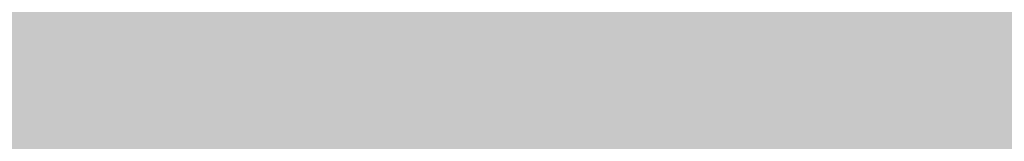
# Model space of a CAD drawing. Units: inches. Extents: x 2083 to 3317, y 1141 to 2115.
# Tile 154 of 256: x 3126.946713 to 3126.955939, y 1263.262504 to 1263.263648. Entities that reach past the tile are written whole.
import ezdxf

# ---------------------------------------------------------------- set-up
doc = ezdxf.new("R2010")
doc.units = ezdxf.units.IN
doc.layers.add('A-ANNO-DIMS', color=2, linetype='Continuous', lineweight=18)
doc.layers.add('A-WALL-PATT', color=251, linetype='Continuous', lineweight=13, true_color=0x636466)
doc.styles.get("Standard").update_dxf_attribs({"font": 'arial.ttf'})
doc.dimstyles.new('ISO-25', dxfattribs={"dimtxt": 12, "dimasz": 12, "dimexe": 1.25, "dimexo": 0.625, "dimtad": 1, "dimlunit": 3, "dimtxsty": 'Standard', "dimcen": 2.5, "dimadec": 0, "dimazin": 0, "dimtfac": 1, "dimtmove": 0, "dimatfit": 3, "dimfxl": 1, "dimarcsym": 0})

# ---------------------------------------------------------------- blocks, each defined once
blk = doc.blocks.new('*D26')
at = {"layer": 'A-ANNO-DIMS', "color": 0, "lineweight": -2, "transparency": 16777216}
for p, q in [((3088.985844, 1274.915092), (3088.985844, 1270.9519631)), ((3111.2400366, 1274.915092), (3111.2400366, 1270.9519631)), ((3076.985844, 1272.2019631), (2840.262447, 1272.2019631)), ((3111.2400366, 1272.2019631), (3088.985844, 1272.2019631)), ((3123.2400366, 1272.2019631), (3135.2400366, 1272.2019631))]:
    blk.add_line(p, q, dxfattribs=at)
at = {"layer": 'A-ANNO-DIMS', "color": 0, "transparency": 16777216}
for points in [[(3076.985844, 1274.2019631), (3076.985844, 1270.2019631), (3088.985844, 1272.2019631)], [(3123.2400366, 1274.2019631), (3123.2400366, 1270.2019631), (3111.2400366, 1272.2019631)]]:
    blk.add_solid(points, dxfattribs=at)
at = {"layer": 'Defpoints', "color": 0, "transparency": 16777216}
for p in [(3088.985844, 1275.540092), (3111.2400366, 1275.540092), (3088.985844, 1272.2019631)]:
    blk.add_point(p, dxfattribs=at)
at = {"layer": 'A-ANNO-DIMS', "color": 0, "transparency": 16777216, "insert": (2952.6241455, 1279.0316016), "char_height": 12, "attachment_point": 5}
blk.add_mtext('NIGHTSTAND 1\'-10 1/2" TYP.', dxfattribs=at)

msp = doc.modelspace()

# ---------------------------------------------------------------- hatches: boundary and pattern name
at = {"layer": 'A-WALL-PATT'}
h = msp.add_hatch(color=256, dxfattribs=at)
h.dxf.hatch_style = 1
h.paths.add_polyline_path([(3126.9597832, 2020.7613601), (2748.9597832, 2020.7613601), (2604.9597832, 2020.7613601), (2226.9597832, 2020.7613601), (2226.9597832, 1702.7613601), (2466.9597832, 1702.7613601), (2466.9597832, 1582.7613601), (2418.9597832, 1582.7613601), (2418.9597832, 1477.7613601), (2226.9597832, 1477.7613601), (2226.9597832, 1263.2613601), (2544.9597832, 1263.2613601), (2544.9597832, 1411.7613601), (2604.9597832, 1411.7613601), (2685.9597832, 1411.7613601), (2685.9597832, 1420.7613601), (2604.9597832, 1420.7613601), (2604.9597832, 1573.7613601), (2604.9597832, 1702.7613601), (2604.9597832, 2011.7613601), (2748.9597832, 2011.7613601), (2748.9597832, 1702.7613601), (2862.9597832, 1702.7613601), (2862.9597832, 1621.7613601), (2871.9597832, 1621.7613601), (2871.9597832, 1702.7613601), (2883.9597832, 1702.7613601), (2883.9597832, 1706.9394595, -0.026459), (2883.9597832, 1711.7613601), (2757.9597832, 1711.7613601), (2757.9597832, 1807.7613601), (2787.9597832, 1807.7613601), (2787.9597832, 1812.2613601), (2757.9597832, 1812.2613601), (2757.9597832, 2011.7613601), (2877.9597832, 2011.7613601), (2877.9597832, 1812.2613601), (2847.9597832, 1812.2613601), (2847.9597832, 1807.7613601), (2889.8357425, 1807.7613601), (2889.8357425, 1812.2613601), (2882.4597832, 1812.2613601), (2882.4597832, 2011.7613601), (3117.9597832, 2011.7613601), (3117.9597832, 1812.2613601), (2937.8357425, 1812.2613601), (2937.8357425, 1807.7613601), (2995.7097832, 1807.7613601), (2995.7097832, 1796.1176655), (3000.2097832, 1796.1176655), (3000.2097832, 1807.7613601), (3117.9597832, 1807.7613601), (3117.9597832, 1711.7613601), (3000.2097832, 1711.7613601), (3000.2097832, 1760.1176655), (2998.5727047, 1760.1176655, -0.020711), (2995.7097832, 1760.1176655), (2995.7097832, 1711.7613601), (2931.9597832, 1711.7613601), (2931.9597832, 1702.7613601), (3126.9597832, 1702.7613601)])
h.paths.add_polyline_path([(2471.4597832, 2011.7613601), (2471.4597832, 1810.0113601), (2462.7169357, 1810.0113601), (2462.7169357, 1805.5113601), (2505.9597832, 1805.5113601), (2505.9597832, 1810.0113601), (2475.9597832, 1810.0113601), (2475.9597832, 2011.7613601), (2595.9597832, 2011.7613601), (2595.9597832, 1810.0113601), (2565.9597832, 1810.0113601), (2565.9597832, 1805.5113601), (2595.9597832, 1805.5113601), (2595.9597832, 1711.7613601), (2235.9597832, 1711.7613601), (2235.9597832, 1805.5113601), (2353.7097832, 1805.5113601), (2353.7097832, 1796.0541624), (2358.2097832, 1796.0541624), (2358.2097832, 1805.5113601), (2414.7169357, 1805.5113601), (2414.7169357, 1810.0113601), (2235.9597832, 1810.0113601), (2235.9597832, 2011.7613601)], flags=16)
h.paths.add_polyline_path([(2270.2047343, 1994.6100082), (2270.2047343, 1970.6100082), (2246.2047343, 1970.6100082), (2246.2047343, 1994.6100082)], flags=0)
edge = h.paths.add_edge_path(flags=0)
edge.add_ellipse((2332.027391, 1899.7981761), major_axis=(-3.0429938, 3.0429938), ratio=0.16825245, start_angle=-161.3321656, end_angle=-156.3071136, ccw=False)
edge.add_ellipse((2333.0820373, 1898.7435297), major_axis=(-1.0546463, 1.0546463), ratio=0.453532097, start_angle=-123.371019, end_angle=-94.1591066)
edge = h.paths.add_edge_path(flags=0)
edge.add_ellipse((2332.027391, 1968.8762897), major_axis=(3.0429938, 3.0429938), ratio=0.16825245, start_angle=18.6678344, end_angle=23.6928864)
edge.add_spline(control_points=[(2332.9255964, 1970.6911045), (2332.2267681, 1970.3360997), (2330.8937087, 1969.6589054), (2328.4130803, 1970.9321376), (2327.2039345, 1967.7487119), (2324.7095965, 1969.9555886), (2322.5328223, 1967.012354), (2320.0128462, 1971.2958124), (2317.6803077, 1968.1578449), (2316.0405263, 1967.1020468), (2315.4269045, 1966.8096022)], knot_values=[0, 0, 0, 0, 2.267059, 4.324559, 6.685584, 8.878641, 11.121502, 14.300359, 17.755284, 19.732645, 19.732645, 19.732645, 19.732645], degree=3, periodic=0)
edge.add_ellipse((2332.027391, 1968.8762897), major_axis=(3.0429938, 3.0429938), ratio=0.16825245, start_angle=18.6678344, end_angle=23.6928864, ccw=False)
edge.add_ellipse((2333.0820373, 1969.930936), major_axis=(1.0546463, 1.0546463), ratio=0.453532097, start_angle=56.628981, end_angle=85.8408934, ccw=False)
edge = h.paths.add_edge_path(flags=0)
edge.add_spline(control_points=[(2296.4282874, 1967.9879081), (2293.6278045, 1965.3363137), (2287.7036238, 1959.727094), (2299.7438601, 1949.9956993), (2294.5325909, 1935.6685275), (2290.5732281, 1920.6035119), (2293.3941244, 1909.9736911), (2296.1854073, 1904.9665431)], knot_values=[0.099185, 0.099185, 0.099185, 0.099185, 0.345301, 0.619822, 0.982653, 1.386093, 1.810555, 1.810555, 1.810555, 1.810555], degree=3, periodic=0)
edge.add_spline(control_points=[(2296.1854073, 1904.9665431), (2297.3835817, 1902.6193002), (2298.0009694, 1901.9493116), (2298.5529698, 1901.4681549)], knot_values=[0.006246, 0.006246, 0.006246, 0.006246, 0.055476, 0.055476, 0.055476, 0.055476], degree=3, periodic=0)
edge.add_spline(control_points=[(2298.5529698, 1901.4681549), (2297.2586121, 1900.9232238), (2295.2252939, 1900.2321257), (2293.0602287, 1900.6142053), (2292.1014227, 1900.788415), (2292.0895776, 1900.790568)], knot_values=[0.312835, 0.312835, 0.312835, 0.312835, 0.40178, 0.474987, 0.475903, 0.475903, 0.475903, 0.475903], degree=3, periodic=0)
edge.add_arc((2292.7936464, 1904.6641088), 3.9370079, 215.4208969, 259.6981795, ccw=False)
edge.add_spline(control_points=[(2289.5853139, 1902.3823039), (2289.4766524, 1902.5350874), (2289.3684805, 1902.6880353), (2289.2608648, 1902.8411699)], knot_values=[0.102872, 0.102872, 0.102872, 0.102872, 0.116896, 0.116896, 0.116896, 0.116896], degree=3, periodic=0)
edge.add_spline(control_points=[(2289.2608648, 1902.8411699), (2288.6866042, 1902.5501922), (2287.6400477, 1902.0199025), (2285.8813368, 1901.8739536), (2283.8529717, 1901.5043521), (2281.7199871, 1899.7105375), (2278.4669913, 1899.492942), (2276.1571361, 1901.8832022), (2272.2589526, 1899.8040711), (2267.7776054, 1901.8431828), (2262.2438819, 1900.1840326), (2257.414927, 1901.7820606), (2254.318374, 1900.7261196), (2253.1782849, 1900.3373431)], knot_values=[0, 0, 0, 0, 1.907977, 3.477176, 5.261074, 7.972851, 11.680248, 13.717921, 16.939592, 22.789562, 27.502503, 33.595215, 37.145618, 37.145618, 37.145618, 37.145618], degree=3, periodic=0)
edge.add_line((2253.1782849, 1900.3373431), (2250.2442397, 1902.8411699))
edge.add_line((2250.2442397, 1902.8411699), (2250.2442397, 1965.8332959))
edge.add_line((2250.2442397, 1965.8332959), (2253.1782849, 1968.3371226))
edge.add_spline(control_points=[(2253.1782849, 1968.3371226), (2254.318374, 1967.9483462), (2257.414927, 1966.8924051), (2262.2438819, 1968.4904332), (2267.7776054, 1966.8312829), (2271.5267301, 1968.5372172), (2273.8759143, 1967.8282895), (2274.2067012, 1967.7276424)], knot_values=[0, 0, 0, 0, 0.09018, 0.244935, 0.364644, 0.513233, 0.537855, 0.537855, 0.537855, 0.537855], degree=3, periodic=0)
edge.add_arc((2274.3528869, 1963.7933495), 3.9370079, 72.0511336, 92.1279492, ccw=False)
edge.add_arc((2281.2969331, 1985.2300027), 18.5962982, 252.05113361, 288.56572166)
edge.add_arc((2292.3167172, 1956.0288805), 12.6460805, 71.02678788, 113.77821843, ccw=False)
edge = h.paths.add_edge_path(flags=0)
edge.add_spline(control_points=[(2274.8994147, 1951.8561946), (2275.066156, 1951.6165924), (2275.2326866, 1951.3765878), (2275.3979871, 1951.1358545)], knot_values=[1.409916, 1.409916, 1.409916, 1.409916, 1.43159, 1.43159, 1.43159, 1.43159], degree=3, periodic=0)
edge.add_spline(control_points=[(2275.3979871, 1951.1358545), (2275.7921055, 1950.5618854), (2276.1792311, 1949.9837745), (2276.5455462, 1949.3971029)], knot_values=[1.358238, 1.358238, 1.358238, 1.358238, 1.409916, 1.409916, 1.409916, 1.409916], degree=3, periodic=0)
edge.add_line((2276.5455462, 1949.3971029), (2277.437289, 1947.8621847))
edge.add_spline(control_points=[(2277.437289, 1947.8621847), (2276.3038341, 1945.6731147), (2274.6396979, 1942.4268817), (2274.631615, 1938.0938998), (2272.7991237, 1930.8515498), (2274.3564261, 1943.8970461), (2275.9476814, 1947.9233558), (2276.5455462, 1949.3971029)], knot_values=[0.005632, 0.005632, 0.005632, 0.005632, 0.186014, 0.266002, 0.357087, 0.59639, 0.739732, 0.739732, 0.739732, 0.739732], degree=3, periodic=0)
edge.add_spline(control_points=[(2276.5455462, 1949.3971029), (2276.1792311, 1949.9837745), (2275.7921055, 1950.5618854), (2275.3979871, 1951.1358545)], knot_values=[1.358238, 1.358238, 1.358238, 1.358238, 1.409916, 1.409916, 1.409916, 1.409916], degree=3, periodic=0)
edge.add_spline(control_points=[(2275.3979871, 1951.1358545), (2274.9425002, 1950.0804523), (2274.2077604, 1948.0252718), (2273.9346018, 1944.8514774), (2272.4685341, 1937.6274891), (2273.4662155, 1945.6964663), (2274.7006154, 1951.0594725), (2274.8994147, 1951.8561946)], knot_values=[0.104364, 0.104364, 0.104364, 0.104364, 0.189636, 0.269624, 0.36071, 0.600013, 0.644622, 0.644622, 0.644622, 0.644622], degree=3, periodic=0)
h.paths.add_polyline_path([(2269.1675139, 1963.1275729, -0.357527), (2268.170633, 1960.9763695, -0.092561), (2268.170633, 1939.4363249, -0.357527), (2269.1675139, 1937.2851215, -0.357527), (2267.0163105, 1938.2820024, -0.164785), (2254.6855813, 1938.2820024, -0.357527), (2252.5343779, 1937.2851215, -0.357527), (2253.5312587, 1939.4363249, -0.092561), (2253.5312587, 1960.9763695, -0.357527), (2252.5343779, 1963.1275729, -0.357527), (2254.6855813, 1962.130692, -0.164785), (2267.0163105, 1962.130692, -0.357527)], flags=0)
h.paths.add_polyline_path([(2248.8740679, 1967.8017998), (2248.8740679, 1957.0277095), (2249.4577833, 1957.0277095), (2249.4577833, 1911.6467562), (2248.8740679, 1911.6467562), (2248.8740679, 1900.8726659), (2246.5118632, 1900.8726659, 0.197327), (2244.1496584, 1902.4568734), (2244.1496584, 1966.2175923, 0.197327), (2246.5118632, 1967.8017998)], flags=0)
h.paths.add_polyline_path([(2269.1675139, 1931.3893442, -0.357527), (2268.170633, 1929.2381408, -0.092561), (2268.170633, 1907.6980962, -0.357527), (2269.1675139, 1905.5468928, -0.357527), (2267.0163105, 1906.5437737, -0.164785), (2254.6855813, 1906.5437737, -0.357527), (2252.5343779, 1905.5468928, -0.357527), (2253.5312587, 1907.6980962, -0.092561), (2253.5312587, 1929.2381408, -0.357527), (2252.5343779, 1931.3893442, -0.357527), (2254.6855813, 1930.3924634, -0.164785), (2267.0163105, 1930.3924634, -0.357527)], flags=0)
edge = h.paths.add_edge_path(flags=0)
edge.add_spline(control_points=[(2276.1968578, 1906.7237016), (2276.1681442, 1909.0289278), (2276.1140492, 1913.371852), (2270.5984171, 1924.9249783), (2273.9051746, 1919.0127787), (2275.9217115, 1916.2620626), (2275.4745699, 1912.4021495), (2277.2578735, 1910.3806206), (2276.6960436, 1908.2250358), (2276.6462176, 1906.8130226), (2276.6178249, 1906.0084068)], knot_values=[0, 0, 0, 0, 8.61026, 16.221274, 18.843057, 23.804898, 27.440828, 29.356102, 31.203478, 33.650687, 33.650687, 33.650687, 33.650687], degree=3, periodic=0)
edge.add_spline(control_points=[(2276.6178249, 1906.0084068), (2276.6233131, 1905.6241436), (2276.4977381, 1904.6286608), (2275.4417789, 1903.8547251), (2274.9373144, 1903.0804497), (2274.8590804, 1902.8411699)], knot_values=[0.156488, 0.156488, 0.156488, 0.156488, 0.184398, 0.231376, 0.250598, 0.250598, 0.250598, 0.250598], degree=3, periodic=0)
edge.add_line((2274.8590804, 1902.8411699), (2276.50598, 1902.8411699))
edge.add_spline(control_points=[(2276.50598, 1902.8411699), (2276.7883084, 1903.0849395), (2277.6650711, 1904.1251958), (2278.2495378, 1904.340738), (2277.6538719, 1908.5273866), (2278.15567, 1906.2278078), (2278.100464, 1905.2859484), (2278.8466748, 1904.0690054), (2277.8567853, 1903.4149482), (2277.8741909, 1902.9910497), (2277.9035616, 1902.8411699)], knot_values=[0.059574, 0.059574, 0.059574, 0.059574, 0.080753, 0.103741, 0.16972, 0.176036, 0.207137, 0.240474, 0.262341, 0.27366, 0.27366, 0.27366, 0.27366], degree=3, periodic=0)
edge.add_line((2277.9035616, 1902.8411699), (2280.0298255, 1902.8411699))
edge.add_spline(control_points=[(2280.0298255, 1902.8411699), (2279.8882214, 1903.088398), (2279.4992571, 1903.9815512), (2280.1522839, 1905.9393491), (2278.103615, 1909.6577572), (2279.7623946, 1907.185285), (2280.3279002, 1904.8748608), (2280.4851086, 1903.4895904), (2281.4632687, 1903.2494323), (2281.7583431, 1902.9364967), (2281.8340361, 1902.8411699)], knot_values=[0.013856, 0.013856, 0.013856, 0.013856, 0.034874, 0.088867, 0.107879, 0.126738, 0.158714, 0.193757, 0.217487, 0.226722, 0.226722, 0.226722, 0.226722], degree=3, periodic=0)
edge.add_spline(control_points=[(2281.8340361, 1902.8411699), (2281.7875348, 1902.8267029), (2281.6470224, 1902.7829881), (2281.3955272, 1902.85949), (2281.088077, 1902.9852418), (2280.7206826, 1903.060902), (2280.3334513, 1903.0257257), (2280.1247668, 1902.898879), (2280.0298255, 1902.8411699)], knot_values=[0, 0, 0, 0, 0.14413, 0.435517, 0.749276, 1.153046, 1.548371, 1.878348, 1.878348, 1.878348, 1.878348], degree=3, periodic=0)
edge.add_line((2280.0298255, 1902.8411699), (2277.9035616, 1902.8411699))
edge.add_spline(control_points=[(2277.9035616, 1902.8411699), (2277.892855, 1902.7958553), (2277.865396, 1902.6796374), (2277.6074793, 1902.6874828), (2277.2740503, 1902.8006999), (2276.8379209, 1902.6197745), (2276.5838074, 1902.7892611), (2276.50598, 1902.8411699)], knot_values=[0, 0, 0, 0, 0.127189, 0.326199, 0.628009, 1.24357, 1.515331, 1.515331, 1.515331, 1.515331], degree=3, periodic=0)
edge.add_line((2276.50598, 1902.8411699), (2274.8590804, 1902.8411699))
edge.add_spline(control_points=[(2274.8590804, 1902.8411699), (2274.8144367, 1902.8985868), (2274.7251297, 1903.013446), (2274.4934765, 1903.1189684), (2274.2442854, 1902.9605386), (2273.9371207, 1903.1849416), (2273.6140395, 1902.9831428), (2273.4083164, 1902.8830449), (2273.322254, 1902.8411699)], knot_values=[0, 0, 0, 0, 0.21843, 0.436957, 0.687977, 0.990379, 1.398396, 1.69185, 1.69185, 1.69185, 1.69185], degree=3, periodic=0)
edge.add_spline(control_points=[(2273.322254, 1902.8411699), (2273.6167403, 1903.445692), (2274.2739977, 1904.5382529), (2276.0272387, 1904.5737017), (2276.2069634, 1906.5836372), (2276.1968578, 1906.7237016)], knot_values=[0.012227, 0.012227, 0.012227, 0.012227, 0.059472, 0.106218, 0.134458, 0.134458, 0.134458, 0.134458], degree=3, periodic=0)
h.paths.add_polyline_path([(2270.7760538, 1897.7898284), (2270.7760538, 1873.7898284), (2246.7760538, 1873.7898284), (2246.7760538, 1897.7898284)], flags=0)
h.paths.add_polyline_path([(2353.7097832, 1760.0050593), (2353.7097832, 1760.0541624), (2358.2097832, 1760.0541624, -0.033729)], flags=0)
h.paths.add_polyline_path([(2321.8191188, 1737.5291862), (2341.9953271, 1737.5291862, -0.414214), (2343.2032727, 1736.3212406), (2343.2032727, 1721.0205964, -0.414214), (2341.9953271, 1719.8126508), (2321.8191188, 1719.8126508, -0.414214), (2320.6111732, 1721.0205964), (2320.6111732, 1736.3212406, -0.414214)], flags=0)
h.paths.add_polyline_path([(2324.2350099, 1736.3212406), (2339.5794359, 1736.3212406, -0.414214), (2341.9953271, 1733.9053494), (2341.9953271, 1725.4497302, -0.414214), (2339.5794359, 1723.033839), (2333.6805885, 1723.033839), (2333.8453172, 1722.0454666, -0.870646), (2335.4253988, 1721.8258934, -0.767327), (2333.922694, 1721.4232449), (2331.2910241, 1721.4232449, -0.767327), (2329.7883193, 1721.8258934, -0.870646), (2331.3684009, 1722.0454666), (2331.5331296, 1723.033839), (2324.2350099, 1723.033839, -0.414214), (2321.8191188, 1725.4497302), (2321.8191188, 1733.9053494, -0.414214)], flags=0)
h.paths.add_polyline_path([(2570.4837892, 1928.6154443), (2589.6837892, 1928.6154443), (2590.1688286, 1928.6154443), (2590.1688286, 1904.9933971), (2570.4837892, 1904.9933971)], flags=0)
h.paths.add_polyline_path([(2574.4473242, 1927.2638215, -1), (2572.8288357, 1927.2638215, -1)], flags=0)
h.paths.add_polyline_path([(2573.0898665, 1926.9408768), (2573.925032, 1927.7760423), (2574.1477428, 1927.5533315), (2573.3125773, 1926.718166)], flags=0)
h.paths.add_polyline_path([(2578.7790648, 1919.7296175, -1), (2571.5916632, 1919.7296175, -1)], flags=0)
h.paths.add_polyline_path([(2578.385364, 1919.7296175, -1), (2571.985364, 1919.7296175, -1)], flags=0)
h.paths.add_polyline_path([(2331.5957638, 1729.4762156, -1), (2333.6179542, 1729.4762156, -1)], flags=0)
h.paths.add_polyline_path([(2578.0342282, 1927.2638215, -1), (2576.4157396, 1927.2638215, -1)], flags=0)
h.paths.add_polyline_path([(2576.6888513, 1927.5310886), (2576.9115621, 1927.7537993), (2577.7467276, 1926.9186339), (2577.5240168, 1926.6959231)], flags=0)
h.paths.add_polyline_path([(2578.1390648, 1909.8595388, -1), (2572.2316632, 1909.8595388, -1)], flags=0)
h.paths.add_polyline_path([(2577.745364, 1909.8595388, -1), (2572.625364, 1909.8595388, -1)], flags=0)
h.paths.add_polyline_path([(2583.7977179, 1927.2638215, -1), (2582.1792294, 1927.2638215, -1)], flags=0)
h.paths.add_polyline_path([(2582.7186487, 1927.7537993), (2583.5538142, 1926.9186339), (2583.3311034, 1926.6959231), (2582.4959379, 1927.5310886)], flags=0)
h.paths.add_polyline_path([(2582.4959379, 1927.5310886), (2582.7186487, 1927.7537993), (2583.5538142, 1926.9186339), (2583.3311034, 1926.6959231)], flags=0)
h.paths.add_polyline_path([(2587.7390648, 1920.5296175, -1), (2581.8316632, 1920.5296175, -1)], flags=0)
h.paths.add_polyline_path([(2587.345364, 1920.5296175, -1), (2582.225364, 1920.5296175, -1)], flags=0)
h.paths.add_polyline_path([(2587.3846219, 1927.2638215, -1), (2585.7661333, 1927.2638215, -1)], flags=0)
h.paths.add_polyline_path([(2586.0819925, 1926.9802469), (2586.917158, 1927.8154124), (2587.1398688, 1927.5927016), (2586.3047033, 1926.7575361)], flags=0)
h.paths.add_polyline_path([(2588.3790648, 1910.6595388, -1), (2581.1916632, 1910.6595388, -1)], flags=0)
h.paths.add_polyline_path([(2587.985364, 1910.6595388, -1), (2581.585364, 1910.6595388, -1)], flags=0)
h.paths.add_polyline_path([(2417.1677288, 1729.4778955), (2437.3439372, 1729.4778955, -0.414214), (2438.5518828, 1728.2699499), (2438.5518828, 1712.9693057, -0.414214), (2437.3439372, 1711.7613601), (2417.1677288, 1711.7613601, -0.414214), (2415.9597832, 1712.9693057), (2415.9597832, 1728.2699499, -0.414214)], flags=0)
h.paths.add_polyline_path([(2419.58362, 1728.2699499), (2434.928046, 1728.2699499, -0.414214), (2437.3439372, 1725.8540587), (2437.3439372, 1717.3984395, -0.414214), (2434.928046, 1714.9825483), (2429.0291985, 1714.9825483), (2429.1939273, 1713.9941758, -0.870646), (2430.7740089, 1713.7746027, -0.767327), (2429.2713041, 1713.3719542), (2426.6396342, 1713.3719542, -0.767327), (2425.1369294, 1713.7746027, -0.870646), (2426.717011, 1713.9941758), (2426.8817397, 1714.9825483), (2419.58362, 1714.9825483, -0.414214), (2417.1677288, 1717.3984395), (2417.1677288, 1725.8540587, -0.414214)], flags=0)
h.paths.add_polyline_path([(2419.58362, 1728.2699499), (2434.928046, 1728.2699499, -0.414214), (2437.3439372, 1725.8540587), (2437.3439372, 1717.3984395, -0.414214), (2434.928046, 1714.9825483), (2429.0291985, 1714.9825483), (2428.3581177, 1719.0090337), (2427.5528206, 1719.0090337), (2426.8817397, 1714.9825483), (2419.58362, 1714.9825483, -0.414214), (2417.1677288, 1717.3984395), (2417.1677288, 1725.8540587, -0.414214)], flags=0)
h.paths.add_polyline_path([(2426.9443739, 1721.4249248, -1), (2428.9665643, 1721.4249248, -1)], flags=0)
h.paths.add_polyline_path([(2475.9597832, 1702.7613601), (2595.9597832, 1702.7613601), (2595.9597832, 1582.7613601), (2475.9597832, 1582.7613601)], flags=16)
h.paths.add_polyline_path([(2427.9597832, 1573.7613601), (2595.9597832, 1573.7613601), (2595.9597832, 1468.7613601), (2595.9597832, 1420.7613601), (2384.4597832, 1420.7613601), (2384.4597832, 1468.7613601), (2427.9597832, 1468.7613601)], flags=16)
h.paths.add_polyline_path([(2379.9597832, 1468.7613601), (2379.9597832, 1420.7613601), (2235.9597832, 1420.7613601), (2235.9597832, 1468.7613601)], flags=16)
h.paths.add_polyline_path([(2317.8159962, 1466.695767), (2337.9922045, 1466.695767, -0.414214), (2339.2001501, 1465.4878214), (2339.2001501, 1450.1871771, -0.414214), (2337.9922045, 1448.9792315), (2317.8159962, 1448.9792315, -0.414214), (2316.6080506, 1450.1871771), (2316.6080506, 1465.4878214, -0.414214)], flags=0)
h.paths.add_polyline_path([(2320.2318874, 1465.4878214), (2335.5763133, 1465.4878214, -0.414214), (2337.9922045, 1463.0719302), (2337.9922045, 1454.616311, -0.414214), (2335.5763133, 1452.2004198), (2329.6774659, 1452.2004198), (2329.8421946, 1451.2120473, -0.870646), (2331.4222762, 1450.9924742, -0.767327), (2329.9195714, 1450.5898257), (2327.2879015, 1450.5898257, -0.767327), (2325.7851967, 1450.9924742, -0.870646), (2327.3652783, 1451.2120473), (2327.530007, 1452.2004198), (2320.2318874, 1452.2004198, -0.414214), (2317.8159962, 1454.616311), (2317.8159962, 1463.0719302, -0.414214)], flags=0)
h.paths.add_polyline_path([(2320.2318874, 1465.4878214), (2335.5763133, 1465.4878214, -0.414214), (2337.9922045, 1463.0719302), (2337.9922045, 1454.616311, -0.414214), (2335.5763133, 1452.2004198), (2329.6774659, 1452.2004198), (2329.006385, 1456.2269051), (2328.2010879, 1456.2269051), (2327.530007, 1452.2004198), (2320.2318874, 1452.2004198, -0.414214), (2317.8159962, 1454.616311), (2317.8159962, 1463.0719302, -0.414214)], flags=0)
h.paths.add_polyline_path([(2327.5926413, 1458.6427963, -1), (2329.6148317, 1458.6427963, -1)], flags=0)
h.paths.add_polyline_path([(2244.4117436, 1433.3404531), (2241.9209449, 1433.3404531, -0.414214), (2240.0178562, 1435.2435418), (2240.0178562, 1440.9528078, -0.414211), (2241.920925, 1442.8558965), (2244.4117436, 1442.8558965, -1.976472)], flags=0)
h.paths.add_polyline_path([(2245.3568884, 1434.3975358, -0.414214), (2245.3568884, 1441.7988138, -2.144098)], flags=0)
h.paths.add_polyline_path([(2535.9597832, 1416.2613601), (2535.9597832, 1272.2613601), (2235.9597832, 1272.2613601), (2235.9597832, 1416.2613601)], flags=16)
h.paths.add_polyline_path([(2260.1195614, 1384.2928413), (2260.1195614, 1362.0386487), (2237.8653688, 1362.0386487), (2237.8653688, 1384.2928413)], flags=0)
edge = h.paths.add_edge_path(flags=0)
edge.add_line((2318.2518466, 1362.0932983), (2318.1457968, 1362.0009726))
edge.add_ellipse((2317.4451158, 1360.4310442), major_axis=(2.8216404, 2.8216404), ratio=0.16825245, start_angle=18.6678344, end_angle=20.9481273, ccw=False)
edge.add_ellipse((2318.4230451, 1361.4089735), major_axis=(0.9779293, 0.9779293), ratio=0.453532097, start_angle=56.628981, end_angle=70.2262012, ccw=False)
edge = h.paths.add_edge_path(flags=0)
edge.add_line((2319.1073699, 1295.5710784), (2319.0150442, 1295.6771282))
edge.add_ellipse((2317.4451158, 1296.3778091), major_axis=(-2.8216404, 2.8216404), ratio=0.16825245, start_angle=-161.3321656, end_angle=-159.0518727, ccw=False)
edge.add_ellipse((2318.4230451, 1295.3998798), major_axis=(-0.9779293, 0.9779293), ratio=0.453532097, start_angle=-123.371019, end_angle=-109.7737988)
edge = h.paths.add_edge_path(flags=0)
edge.add_spline(control_points=[(2284.2103489, 1301.1702189), (2284.5806878, 1300.444719), (2284.8911891, 1299.8920243), (2285.159553, 1299.4610182)], knot_values=[0.039066, 0.039066, 0.039066, 0.039066, 0.055476, 0.055476, 0.055476, 0.055476], degree=3, periodic=0)
edge.add_line((2285.159553, 1299.4610182), (2284.2103489, 1301.1702189))
edge = h.paths.add_edge_path(flags=0)
edge.add_line((2280.4124579, 1297.2980125), (2283.3699905, 1297.0361216))
edge.add_line((2283.3699905, 1297.0361216), (2286.4056902, 1297.9263104))
edge.add_spline(control_points=[(2286.4056902, 1297.9263104), (2285.305487, 1297.4631193), (2284.3447774, 1297.1291508), (2283.3699905, 1297.0361216)], knot_values=[0.394369, 0.394369, 0.394369, 0.394369, 0.475903, 0.475903, 0.475903, 0.475903], degree=3, periodic=0)
edge.add_spline(control_points=[(2283.3699905, 1297.0361216), (2283.2813895, 1297.027666), (2282.316289, 1296.9573356), (2281.3125019, 1297.1344787), (2280.4234414, 1297.2960161), (2280.4124579, 1297.2980125)], knot_values=[0.312835, 0.312835, 0.312835, 0.312835, 0.320246, 0.393453, 0.394369, 0.394369, 0.394369, 0.394369], degree=3, periodic=0)
edge = h.paths.add_edge_path(flags=0)
edge.add_line((2284.4355615, 1359.6072854), (2280.4462909, 1355.328047))
edge.add_line((2280.4462909, 1355.328047), (2279.5799868, 1351.0177544))
edge.add_line((2279.5799868, 1351.0177544), (2282.4129737, 1346.5804327))
edge.add_spline(control_points=[(2282.4129737, 1346.5804327), (2283.1533308, 1345.5892358), (2284.2528957, 1344.0288973), (2284.801037, 1342.3871671), (2284.9351625, 1341.8055443)], knot_values=[1.240098, 1.240098, 1.240098, 1.240098, 1.332892, 1.382712, 1.382712, 1.382712, 1.382712], degree=3, periodic=0)
edge.add_spline(control_points=[(2284.9351625, 1341.8055443), (2285.3191079, 1340.1406002), (2285.2330291, 1338.4092041), (2284.9099384, 1336.6541222)], knot_values=[1.097484, 1.097484, 1.097484, 1.097484, 1.240098, 1.240098, 1.240098, 1.240098], degree=3, periodic=0)
edge.add_spline(control_points=[(2284.9099384, 1336.6541222), (2284.5868478, 1334.8990403), (2284.0267453, 1333.1202725), (2283.4626437, 1331.3605849)], knot_values=[0.95487, 0.95487, 0.95487, 0.95487, 1.097484, 1.097484, 1.097484, 1.097484], degree=3, periodic=0)
edge.add_line((2283.4626437, 1331.3605849), (2281.8903759, 1326.153357))
edge.add_line((2281.8903759, 1326.153357), (2280.7562592, 1321.0560888))
edge.add_line((2280.7562592, 1321.0560888), (2280.2992048, 1316.0019772))
edge.add_line((2280.2992048, 1316.0019772), (2280.7159327, 1310.9500678))
edge.add_line((2280.7159327, 1310.9500678), (2282.0280939, 1305.9721367))
edge.add_line((2282.0280939, 1305.9721367), (2284.2103489, 1301.1702189))
edge.add_spline(control_points=[(2284.2103489, 1301.1702189), (2283.3407305, 1302.7301854), (2282.6119044, 1304.3364933), (2282.0280939, 1305.9721367)], knot_values=[0.099185, 0.099185, 0.099185, 0.099185, 0.241799, 0.241799, 0.241799, 0.241799], degree=3, periodic=0)
edge.add_spline(control_points=[(2282.0280939, 1305.9721367), (2281.4442835, 1307.6077801), (2281.0054886, 1309.2727591), (2280.7159327, 1310.9500678)], knot_values=[0.241799, 0.241799, 0.241799, 0.241799, 0.384413, 0.384413, 0.384413, 0.384413], degree=3, periodic=0)
edge.add_spline(control_points=[(2280.7159327, 1310.9500678), (2280.4332411, 1312.5876134), (2280.2893863, 1314.2769594), (2280.2988938, 1315.9620324), (2280.2992048, 1316.0019772)], knot_values=[0.384413, 0.384413, 0.384413, 0.384413, 0.523647, 0.527028, 0.527028, 0.527028, 0.527028], degree=3, periodic=0)
edge.add_spline(control_points=[(2280.2992048, 1316.0019772), (2280.3123257, 1317.6869552), (2280.4778706, 1319.3679256), (2280.7562592, 1321.0560888)], knot_values=[0.527028, 0.527028, 0.527028, 0.527028, 0.669642, 0.669642, 0.669642, 0.669642], degree=3, periodic=0)
edge.add_spline(control_points=[(2280.7562592, 1321.0560888), (2281.0346478, 1322.7442519), (2281.4258801, 1324.4396079), (2281.8903759, 1326.153357)], knot_values=[0.669642, 0.669642, 0.669642, 0.669642, 0.812256, 0.812256, 0.812256, 0.812256], degree=3, periodic=0)
edge.add_spline(control_points=[(2281.8903759, 1326.153357), (2282.2643834, 1327.5332507), (2282.7878702, 1329.2618097), (2283.352751, 1331.0177803), (2283.4626437, 1331.3605849)], knot_values=[0.812256, 0.812256, 0.812256, 0.812256, 0.927087, 0.95487, 0.95487, 0.95487, 0.95487], degree=3, periodic=0)
edge.add_line((2283.4626437, 1331.3605849), (2284.9099384, 1336.6541222))
edge.add_line((2284.9099384, 1336.6541222), (2284.9351625, 1341.8055443))
edge.add_line((2284.9351625, 1341.8055443), (2282.4129737, 1346.5804327))
edge.add_spline(control_points=[(2282.4129737, 1346.5804327), (2281.2751273, 1348.1037918), (2280.0784467, 1349.5703178), (2279.5799868, 1351.0177544)], knot_values=[1.382712, 1.382712, 1.382712, 1.382712, 1.525326, 1.525326, 1.525326, 1.525326], degree=3, periodic=0)
edge.add_spline(control_points=[(2279.5799868, 1351.0177544), (2279.4432818, 1351.4147209), (2279.1363124, 1352.856922), (2279.7351897, 1354.2903851), (2280.4462909, 1355.328047)], knot_values=[1.525326, 1.525326, 1.525326, 1.525326, 1.564439, 1.667941, 1.667941, 1.667941, 1.667941], degree=3, periodic=0)
edge.add_spline(control_points=[(2280.4462909, 1355.328047), (2281.4261132, 1356.7578354), (2282.9308373, 1358.1825604), (2284.4355615, 1359.6072854)], knot_values=[1.667941, 1.667941, 1.667941, 1.667941, 1.810555, 1.810555, 1.810555, 1.810555], degree=3, periodic=0)
edge.add_arc((2280.6230749, 1348.518181), 11.7261796, 71.02678788, 113.77821843)
edge.add_arc((2270.4048917, 1375.5951559), 17.2435667, 252.05113361, 288.56572166, ccw=False)
edge.add_arc((2263.9659692, 1355.7178471), 3.6506221, 72.0511336, 92.1279492)
edge.add_arc((2263.9659692, 1355.7178471), 3.6506221, 92.1279492, 177.98513)
edge.add_spline(control_points=[(2260.3176041, 1355.8461989), (2260.2604169, 1354.2206683), (2260.551278, 1350.1865469), (2262.9993445, 1346.7662507), (2264.4727415, 1344.6490245)], knot_values=[1.43159, 1.43159, 1.43159, 1.43159, 1.564144, 1.770695, 1.770695, 1.770695, 1.770695], degree=3, periodic=0)
edge.add_line((2264.4727415, 1344.6490245), (2264.9355904, 1343.9825301))
edge.add_spline(control_points=[(2263.8010444, 1340.2481052), (2263.8432379, 1340.5140884), (2264.0672444, 1341.7564652), (2264.5126928, 1343.0024532), (2264.9350468, 1343.9810834)], knot_values=[0.53657, 0.53657, 0.53657, 0.53657, 0.559349, 0.644622, 0.644622, 0.644622, 0.644622], degree=3, periodic=0)
edge.add_spline(control_points=[(2264.9350468, 1343.9810834), (2265.1177715, 1343.7149747), (2265.2988751, 1343.4479058), (2265.4767562, 1343.1793646)], knot_values=[1.384077, 1.384077, 1.384077, 1.384077, 1.409916, 1.409916, 1.409916, 1.409916], degree=3, periodic=0)
edge.add_spline(control_points=[(2265.4767562, 1343.1793646), (2265.6546373, 1342.9108234), (2265.8292958, 1342.64081), (2265.9991301, 1342.368812)], knot_values=[1.358238, 1.358238, 1.358238, 1.358238, 1.384077, 1.384077, 1.384077, 1.384077], degree=3, periodic=0)
edge.add_line((2265.9991301, 1342.368812), (2266.8260057, 1340.9455468))
edge.add_spline(control_points=[(2266.8260057, 1340.9455468), (2268.894401, 1337.0896912), (2271.3981727, 1325.8430009), (2270.5161644, 1310.5685568), (2275.9193759, 1301.860609), (2277.7895113, 1299.1994495)], knot_values=[0.116896, 0.116896, 0.116896, 0.116896, 0.472987, 1.050969, 1.313793, 1.313793, 1.313793, 1.313793], degree=3, periodic=0)
edge.add_spline(control_points=[(2277.7895113, 1299.1994495), (2277.8394051, 1299.1284519), (2277.8894277, 1299.0574975), (2277.9395717, 1298.9865839)], knot_values=[0.109884, 0.109884, 0.109884, 0.109884, 0.116896, 0.116896, 0.116896, 0.116896], degree=3, periodic=0)
edge.add_line((2277.9395717, 1298.9865839), (2277.7888489, 1299.1991139))
edge.add_spline(control_points=[(2277.7888489, 1299.1991139), (2277.2565819, 1298.9294144), (2276.2863504, 1298.4379024), (2275.0393517, 1298.3344186), (2274.3833299, 1298.2388951), (2274.2152543, 1298.209338)], knot_values=[33.12187, 33.12187, 33.12187, 33.12187, 35.029056, 36.598255, 37.144827, 37.144827, 37.144827, 37.144827], degree=3, periodic=0)
edge.add_line((2274.2152543, 1298.209338), (2273.073147, 1297.8929607))
edge.add_spline(control_points=[(2273.073147, 1297.8929607), (2272.3229363, 1297.579784), (2271.0391507, 1296.5105078), (2269.2483948, 1296.2260622), (2268.4231004, 1296.3746543)], knot_values=[26.532584, 26.532584, 26.532584, 26.532584, 29.198919, 31.839101, 31.839101, 31.839101, 31.839101], degree=3, periodic=0)
edge.add_line((2268.4231004, 1296.3746543), (2263.8785014, 1297.4575338))
edge.add_spline(control_points=[(2263.8785014, 1297.4575338), (2263.5560769, 1297.3594345), (2261.8603064, 1296.8386943), (2260.2387805, 1297.2824073), (2258.9334543, 1297.5164611)], knot_values=[15.919551, 15.919551, 15.919551, 15.919551, 16.939592, 21.226067, 21.226067, 21.226067, 21.226067], degree=3, periodic=0)
edge.add_line((2258.9334543, 1297.5164611), (2254.0552332, 1297.3290098))
edge.add_spline(control_points=[(2254.0552332, 1297.3290098), (2253.7555255, 1297.295815), (2252.1136834, 1297.1651738), (2250.4618687, 1297.5442209), (2249.1296862, 1297.6678818)], knot_values=[5.306517, 5.306517, 5.306517, 5.306517, 6.276435, 10.613034, 10.613034, 10.613034, 10.613034], degree=3, periodic=0)
edge.add_line((2249.1296862, 1297.6678818), (2244.3316495, 1296.8777561))
edge.add_line((2244.3316495, 1296.8777561), (2241.6110326, 1299.1994495))
edge.add_line((2241.6110326, 1299.1994495), (2241.6110326, 1357.6094038))
edge.add_line((2241.6110326, 1357.6094038), (2244.3316495, 1359.9310973))
edge.add_line((2244.3316495, 1359.9310973), (2252.7288228, 1359.5426917))
edge.add_spline(control_points=[(2252.7288228, 1359.5426917), (2252.8709387, 1359.5464396), (2253.3057402, 1359.5481716), (2253.7398447, 1359.5142744), (2254.0317419, 1359.4824261)], knot_values=[0.233291, 0.233291, 0.233291, 0.233291, 0.244935, 0.268927, 0.268927, 0.268927, 0.268927], degree=3, periodic=0)
edge.add_line((2254.0317419, 1359.4824261), (2259.5871899, 1359.4163899))
edge.add_spline(control_points=[(2259.5871899, 1359.4163899), (2260.6770676, 1359.6285026), (2262.0731971, 1359.8970025), (2263.5236925, 1359.4592776), (2263.8304173, 1359.3659518)], knot_values=[0.422516, 0.422516, 0.422516, 0.422516, 0.513233, 0.537855, 0.537855, 0.537855, 0.537855], degree=3, periodic=0)
edge.add_arc((2263.9659692, 1355.7178471), 3.6506221, 72.0511336, 92.1279492, ccw=False)
edge.add_arc((2270.4048917, 1375.5951559), 17.2435667, 252.05113361, 288.56572166)
edge.add_arc((2280.6230749, 1348.518181), 11.7261796, 71.02678788, 113.77821843, ccw=False)
h.paths.add_polyline_path([(2240.3405298, 1359.4347149), (2240.3405298, 1349.4443532), (2240.8817846, 1349.4443532), (2240.8817846, 1307.3645001), (2240.3405298, 1307.3645001), (2240.3405298, 1297.3741385), (2238.1501565, 1297.3741385, 0.197327), (2235.9597832, 1298.8431076), (2235.9597832, 1357.9657458, 0.197327), (2238.1501565, 1359.4347149)], flags=0)
h.paths.add_polyline_path([(2259.1577904, 1355.1005005, -0.357527), (2258.2334246, 1353.1057799, -0.092561), (2258.2334246, 1333.1326007, -0.357527), (2259.1577904, 1331.1378801, -0.357527), (2257.1630698, 1332.0622458, -0.164785), (2245.7293022, 1332.0622458, -0.357527), (2243.7345816, 1331.1378801, -0.357527), (2244.6589474, 1333.1326007, -0.092561), (2244.6589474, 1353.1057799, -0.357527), (2243.7345816, 1355.1005005, -0.357527), (2245.7293022, 1354.1761347, -0.164785), (2257.1630698, 1354.1761347, -0.357527)], flags=0)
edge = h.paths.add_edge_path(flags=0)
edge.add_line((2265.9991301, 1342.368812), (2266.8260057, 1340.9455468))
edge.add_line((2266.8260057, 1340.9455468), (2265.3075567, 1337.8140664))
edge.add_line((2265.3075567, 1337.8140664), (2264.358232, 1334.6529388))
edge.add_line((2264.358232, 1334.6529388), (2264.2620123, 1333.7997046))
edge.add_spline(control_points=[(2264.2620123, 1333.7997046), (2264.2083565, 1333.187055), (2264.1620602, 1332.3655252), (2264.0071444, 1331.4139326), (2263.9690487, 1331.2018338)], knot_values=[0.464444, 0.464444, 0.464444, 0.464444, 0.516691, 0.531608, 0.531608, 0.531608, 0.531608], degree=3, periodic=0)
edge.add_spline(control_points=[(2263.9690487, 1331.2018338), (2263.7745349, 1330.1188727), (2263.4243703, 1328.7908386), (2263.2574202, 1328.5306516), (2263.2340282, 1328.5146115)], knot_values=[0.372682, 0.372682, 0.372682, 0.372682, 0.44885, 0.464444, 0.464444, 0.464444, 0.464444], degree=3, periodic=0)
edge.add_spline(control_points=[(2263.2340282, 1328.5146115), (2263.096382, 1328.4202271), (2263.1311696, 1329.3014765), (2263.2749528, 1330.6157493)], knot_values=[0.280919, 0.280919, 0.280919, 0.280919, 0.372682, 0.372682, 0.372682, 0.372682], degree=3, periodic=0)
edge.add_spline(control_points=[(2263.2749528, 1330.6157493), (2263.4187361, 1331.930022), (2263.6715151, 1333.677318), (2263.9698519, 1335.3150268)], knot_values=[0.189157, 0.189157, 0.189157, 0.189157, 0.280919, 0.280919, 0.280919, 0.280919], degree=3, periodic=0)
edge.add_spline(control_points=[(2263.9698519, 1335.3150268), (2264.1004958, 1336.0321917), (2264.4187827, 1337.6219113), (2264.7548476, 1338.8644304), (2264.9474193, 1339.4911244)], knot_values=[0.097394, 0.097394, 0.097394, 0.097394, 0.137578, 0.189157, 0.189157, 0.189157, 0.189157], degree=3, periodic=0)
edge.add_spline(control_points=[(2264.9474193, 1339.4911244), (2265.2900171, 1340.6060546), (2265.6442376, 1341.4939958), (2265.9991301, 1342.368812)], knot_values=[0.005632, 0.005632, 0.005632, 0.005632, 0.097394, 0.097394, 0.097394, 0.097394], degree=3, periodic=0)
h.paths.add_polyline_path([(2259.1577904, 1325.6709733, -0.357527), (2258.2334246, 1323.6762527, -0.092561), (2258.2334246, 1303.7030735, -0.357527), (2259.1577904, 1301.7083529, -0.357527), (2257.1630698, 1302.6327186, -0.164785), (2245.7293022, 1302.6327186, -0.357527), (2243.7345816, 1301.7083529, -0.357527), (2244.6589474, 1303.7030735, -0.092561), (2244.6589474, 1323.6762527, -0.357527), (2243.7345816, 1325.6709733, -0.357527), (2245.7293022, 1324.7466075, -0.164785), (2257.1630698, 1324.7466075, -0.357527)], flags=0)
edge = h.paths.add_edge_path(flags=0)
edge.add_spline(control_points=[(2261.7089377, 1317.3114208), (2261.6794818, 1317.4175798), (2261.7618581, 1317.3885347), (2262.4907358, 1316.0898725), (2262.962185, 1315.3008975)], knot_values=[14.955861, 14.955861, 14.955861, 14.955861, 16.221274, 18.694826, 18.694826, 18.694826, 18.694826], degree=3, periodic=0)
edge.add_spline(control_points=[(2262.962185, 1315.3008975), (2262.9904374, 1315.2536169), (2263.7020958, 1314.0673762), (2264.3489834, 1313.1271533), (2264.7300545, 1312.1641544)], knot_values=[18.694826, 18.694826, 18.694826, 18.694826, 18.843057, 22.433791, 22.433791, 22.433791, 22.433791], degree=3, periodic=0)
edge.add_spline(control_points=[(2264.7300545, 1312.1641544), (2264.8755649, 1311.7964373), (2265.1768733, 1310.7698073), (2265.1430689, 1309.5592623), (2265.2477363, 1308.8241926)], knot_values=[22.433791, 22.433791, 22.433791, 22.433791, 23.804898, 26.172756, 26.172756, 26.172756, 26.172756], degree=3, periodic=0)
edge.add_line((2265.2477363, 1308.8241926), (2265.8507741, 1307.1718879))
edge.add_spline(control_points=[(2265.8507741, 1307.1718879), (2266.0650246, 1306.8216779), (2266.3843872, 1306.3322461), (2266.4244001, 1305.7805489), (2266.4203688, 1305.6112163)], knot_values=[28.062562, 28.062562, 28.062562, 28.062562, 29.356102, 29.911721, 29.911721, 29.911721, 29.911721], degree=3, periodic=0)
edge.add_spline(control_points=[(2266.4203688, 1305.6112163), (2266.4161162, 1305.4325896), (2266.393999, 1305.2499979), (2266.3647773, 1305.0658571)], knot_values=[29.911721, 29.911721, 29.911721, 29.911721, 30.497837, 30.497837, 30.497837, 30.497837], degree=3, periodic=0)
edge.add_line((2266.3647773, 1305.0658571), (2266.0661511, 1302.1362954))
edge.add_spline(control_points=[(2266.0661511, 1302.1362954), (2266.0712401, 1301.7799843), (2265.9980761, 1301.1999847), (2265.6632664, 1300.7589613), (2265.5089084, 1300.5858824)], knot_values=[0.156488, 0.156488, 0.156488, 0.156488, 0.184398, 0.203543, 0.203543, 0.203543, 0.203543], degree=3, periodic=0)
edge.add_line((2265.5089084, 1300.5858824), (2264.4353411, 1299.1994495))
edge.add_line((2264.4353411, 1299.1994495), (2265.962442, 1299.1994495))
edge.add_line((2265.962442, 1299.1994495), (2267.3359898, 1301.1752758))
edge.add_line((2267.3359898, 1301.1752758), (2267.3116668, 1301.9862366))
edge.add_spline(control_points=[(2267.3116668, 1301.9862366), (2267.261111, 1302.8623959), (2267.1602121, 1303.7371316), (2267.2714865, 1303.3258962)], knot_values=[0.126229, 0.126229, 0.126229, 0.126229, 0.166617, 0.166617, 0.166617, 0.166617], degree=3, periodic=0)
edge.add_spline(control_points=[(2267.2714865, 1303.3258962), (2267.2800347, 1303.2943047), (2267.3097851, 1303.1753659), (2267.3734504, 1302.8836084), (2267.4061233, 1302.6828291), (2267.4179259, 1302.6010251)], knot_values=[0.166617, 0.166617, 0.166617, 0.166617, 0.16972, 0.176036, 0.180765, 0.180765, 0.180765, 0.180765], degree=3, periodic=0)
edge.add_spline(control_points=[(2267.7438914, 1300.9875045), (2267.6875832, 1301.1509426), (2267.4805198, 1301.6566644), (2267.4837514, 1302.1447877), (2267.4179259, 1302.6010251)], knot_values=[0.180765, 0.180765, 0.180765, 0.180765, 0.193767, 0.220139, 0.220139, 0.220139, 0.220139], degree=3, periodic=0)
edge.add_line((2267.4179259, 1302.6010251), (2267.7438914, 1300.9875045))
edge.add_spline(control_points=[(2267.7438914, 1300.9875045), (2267.8319608, 1300.7318778), (2267.9320205, 1300.3099042), (2267.5548409, 1299.9745185), (2267.429366, 1299.8292073)], knot_values=[0.220139, 0.220139, 0.220139, 0.220139, 0.240474, 0.25489, 0.25489, 0.25489, 0.25489], degree=3, periodic=0)
edge.add_line((2267.429366, 1299.8292073), (2267.2583608, 1299.1994495))
edge.add_line((2267.2583608, 1299.1994495), (2269.229956, 1299.1994495))
edge.add_spline(control_points=[(2269.229956, 1299.1994495), (2269.0986525, 1299.4286938), (2268.842774, 1300.0162509), (2269.0115749, 1300.9159235), (2268.9467957, 1301.6607397)], knot_values=[0.013856, 0.013856, 0.013856, 0.013856, 0.034874, 0.067073, 0.067073, 0.067073, 0.067073], degree=3, periodic=0)
edge.add_line((2268.9467957, 1301.6607397), (2268.4315815, 1303.6031089))
edge.add_spline(control_points=[(2268.4315815, 1303.6031089), (2268.1755957, 1304.1923747), (2267.5962136, 1305.2512977), (2268.0406981, 1304.6232098), (2268.2513938, 1304.2824205)], knot_values=[0.090155, 0.090155, 0.090155, 0.090155, 0.107879, 0.120289, 0.120289, 0.120289, 0.120289], degree=3, periodic=0)
edge.add_spline(control_points=[(2268.2513938, 1304.2824205), (2268.3608818, 1304.1053294), (2269.0577527, 1302.9179833), (2269.382691, 1301.5904186), (2269.5214051, 1300.7759312), (2269.5752202, 1300.5557836)], knot_values=[0.120289, 0.120289, 0.120289, 0.120289, 0.126738, 0.158714, 0.173506, 0.173506, 0.173506, 0.173506], degree=3, periodic=0)
edge.add_line((2269.5752202, 1300.5557836), (2270.6857984, 1299.4212579))
edge.add_spline(control_points=[(2270.6857984, 1299.4212579), (2270.7672206, 1299.3572512), (2270.8378523, 1299.2814011), (2270.9029248, 1299.1994495)], knot_values=[0.21816, 0.21816, 0.21816, 0.21816, 0.226722, 0.226722, 0.226722, 0.226722], degree=3, periodic=0)
edge.add_line((2270.9372012, 1299.1929131), (2270.9029248, 1299.1994495))
edge.add_spline(control_points=[(2270.9029248, 1299.1994495), (2270.8598061, 1299.1860349), (2270.7295148, 1299.1455), (2270.4963139, 1299.216437), (2270.2716612, 1299.3083234), (2270.1210168, 1299.3479612), (2270.0633386, 1299.3595566)], knot_values=[0.939174, 0.939174, 0.939174, 0.939174, 1.083304, 1.374691, 1.68845, 1.878348, 1.878348, 1.878348, 1.878348], degree=3, periodic=0)
edge.add_line((2270.0633386, 1299.3595566), (2269.229956, 1299.1994495))
edge.add_line((2269.229956, 1299.1994495), (2267.2583608, 1299.1994495))
edge.add_spline(control_points=[(2267.2583608, 1299.1994495), (2267.248433, 1299.1574312), (2267.2229714, 1299.0496673), (2266.9838161, 1299.056942), (2266.8092097, 1299.1162303), (2266.6769047, 1299.1090913), (2266.636531, 1299.1048147)], knot_values=[0.757665, 0.757665, 0.757665, 0.757665, 0.884854, 1.083864, 1.385675, 1.515331, 1.515331, 1.515331, 1.515331], degree=3, periodic=0)
edge.add_spline(control_points=[(2266.636531, 1299.1048147), (2266.4852248, 1299.0887878), (2266.2358066, 1299.0171229), (2266.0346081, 1299.1513168), (2265.962442, 1299.1994495)], knot_values=[0, 0, 0, 0, 0.485905, 0.757665, 0.757665, 0.757665, 0.757665], degree=3, periodic=0)
edge.add_line((2265.962442, 1299.1994495), (2264.4353411, 1299.1994495))
edge.add_line((2264.4353411, 1299.1994495), (2263.8584442, 1299.3671176))
edge.add_spline(control_points=[(2263.8584442, 1299.3671176), (2263.8189433, 1299.3709053), (2263.7795277, 1299.3857212), (2263.7401308, 1299.4015039)], knot_values=[0.845925, 0.845925, 0.845925, 0.845925, 0.978627, 0.978627, 0.978627, 0.978627], degree=3, periodic=0)
edge.add_line((2263.7217862, 1299.3964251), (2263.0103065, 1299.1994495))
edge.add_spline(control_points=[(2263.0103065, 1299.1994495), (2263.2457942, 1299.682859), (2263.5060317, 1300.1281072), (2263.8734943, 1300.4080279)], knot_values=[0.012227, 0.012227, 0.012227, 0.012227, 0.052971, 0.052971, 0.052971, 0.052971], degree=3, periodic=0)
edge.add_spline(control_points=[(2263.8734943, 1300.4080279), (2263.932131, 1300.4526954), (2264.0842429, 1300.5529789), (2264.2551889, 1300.6242227), (2264.3596855, 1300.6647475)], knot_values=[0.052971, 0.052971, 0.052971, 0.052971, 0.059472, 0.069086, 0.069086, 0.069086, 0.069086], degree=3, periodic=0)
edge.add_line((2264.3596855, 1300.6647475), (2265.1418998, 1301.0777737))
edge.add_line((2265.1418998, 1301.0777737), (2265.675806, 1302.7995583))
edge.add_line((2265.675806, 1302.7995583), (2265.5407004, 1305.7040662))
edge.add_line((2265.5407004, 1305.7040662), (2264.8030733, 1309.3277237))
edge.add_line((2264.8030733, 1309.3277237), (2263.0405349, 1314.0917906))
edge.add_spline(control_points=[(2263.0405349, 1314.0917906), (2262.3835724, 1315.6714379), (2261.7959724, 1316.9977489), (2261.7089377, 1317.3114208)], knot_values=[11.216896, 11.216896, 11.216896, 11.216896, 14.955861, 14.955861, 14.955861, 14.955861], degree=3, periodic=0)
h.paths.add_polyline_path([(2871.9597832, 1416.2613601), (2895.910047, 1416.2613601), (2895.910047, 1420.7613601), (2871.9597832, 1420.7613601), (2871.9597832, 1501.7613601), (2862.9597832, 1501.7613601), (2862.9597832, 1420.7613601), (2805.9597832, 1420.7613601), (2805.9597832, 1411.7613601), (2862.9597832, 1411.7613601), (2862.9597832, 1263.2613601), (3126.9597832, 1263.2613601), (3126.9597832, 1411.7613601), (3126.9597832, 1486.7613601), (2943.9597832, 1486.7613601), (2943.9597832, 1477.7613601), (2967.8603109, 1477.7613601), (2967.8603109, 1420.7613601), (2943.910047, 1420.7613601), (2943.910047, 1416.2613601), (3117.9597832, 1416.2613601), (3117.9597832, 1420.7613601), (2972.3603109, 1420.7613601), (2972.3603109, 1477.7613601), (3117.9597832, 1477.7613601), (3117.9597832, 1420.7613601), (3117.9597832, 1272.2613601), (2871.9597832, 1272.2613601)], flags=0)
h.paths.add_polyline_path([(2457.1256256, 1485.9425054), (2527.6026508, 1485.9425054), (2527.6026508, 1537.6357021), (2457.1256256, 1537.6357021)], flags=8)
h.paths.add_polyline_path([(2481.0050583, 1609.9818039), (2590.765818, 1609.9818039), (2590.765818, 1682.0033623), (2481.0050583, 1682.0033623)], flags=8)
h.paths.add_polyline_path([(2483.0850224, 1729.1267835), (2553.5620476, 1729.1267835), (2553.5620476, 1780.8199802), (2483.0850224, 1780.8199802)], flags=8)
h = msp.add_hatch(color=256, dxfattribs=at)
h.dxf.hatch_style = 1
h.paths.add_polyline_path([(3126.9597832, 1486.7613601), (2943.9597832, 1486.7613601), (2943.9597832, 1477.7613601), (2967.8603109, 1477.7613601), (2967.8603109, 1420.7613601), (2943.910047, 1420.7613601), (2943.910047, 1416.2613601), (3117.9597832, 1416.2613601), (3117.9597832, 1420.7613601), (2972.3603109, 1420.7613601), (2972.3603109, 1477.7613601), (3117.9597832, 1477.7613601), (3117.9597832, 1420.7613601), (3117.9597832, 1272.2613601), (2871.9597832, 1272.2613601), (2871.9597832, 1416.2613601), (2895.910047, 1416.2613601), (2895.910047, 1420.7613601), (2871.9597832, 1420.7613601), (2871.9597832, 1501.7613601), (2862.9597832, 1501.7613601), (2862.9597832, 1420.7613601), (2805.9597832, 1420.7613601), (2805.9597832, 1411.7613601), (2862.9597832, 1411.7613601), (2862.9597832, 1263.2613601), (3126.9597832, 1263.2613601), (3126.9597832, 1411.7613601)])

# ---------------------------------------------------------------- dimensions: what is measured, and where the dimension line sits
at = {"layer": 'A-ANNO-DIMS'}
dim = msp.add_linear_dim(base=(3088.985844, 1272.2019631), p1=(3111.2400366, 1275.540092), p2=(3088.985844, 1275.540092), angle=180, text='NIGHTSTAND <> TYP.', dimstyle='ISO-25', override={"dimdec": 1, "dimlfac": 1, "dimrnd": 0, "dimzin": 1, "dimdsep": 46, "dimlunit": 4, "dimfrac": 2}, dxfattribs=at)
dim.commit()
dim.dimension.update_dxf_attribs({"geometry": '*D26', "text_midpoint": (2952.6241455, 1279.0316016)})

doc.saveas('drawing.dxf')
